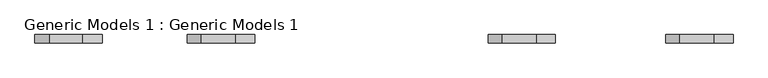
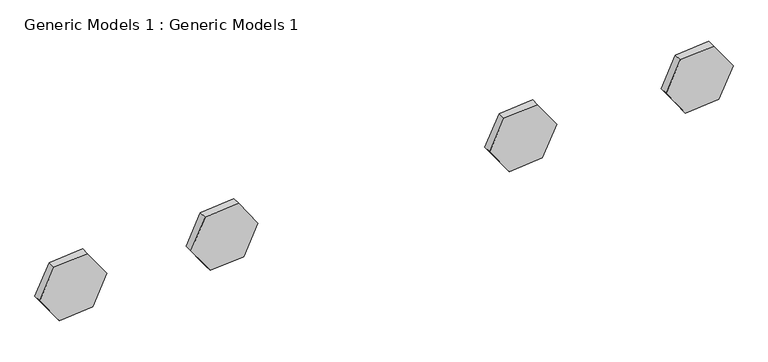
"""IFC4 building model written with IfcOpenShell, lengths in millimetres: proxy geometry, Generic Models 1 : Generic Models 1."""

from ifc_helpers import new_model, si_unit, frame, origin, place, context, project, spatial, polyline, outline, extrude, source, transform, mapped, element, save


def generic_models_1_generic_models_1_2c748ff4(model_context):
    return source(origin(), model_context, "Body", "SweptSolid", [
        extrude(outline(polyline([(1160.0163885, -6657.533371), (607.5311616, -6915.1614634), (108.1760754, -6565.5092678), (161.3062161, -5958.2289798), (713.7914431, -5700.6008875), (1213.1465293, -6050.2530831), (1160.0163885, -6657.533371)])), frame((0.0, -11889.415504, 0.0), z_axis=(0.0, 1.0, 0.0), x_axis=(0.0, 0.0, 1.0)), (0.0, 0.0, 1.0), 152.4),
        extrude(outline(polyline([(1160.0163885, -3914.333371), (607.5311616, -4171.9614634), (108.1760754, -3822.3092678), (161.3062161, -3215.0289798), (713.7914431, -2957.4008875), (1213.1465293, -3307.0530831), (1160.0163885, -3914.333371)])), frame((0.0, -11889.415504, 0.0), z_axis=(0.0, 1.0, 0.0), x_axis=(0.0, 0.0, 1.0)), (0.0, 0.0, 1.0), 152.4),
        extrude(outline(polyline([(1160.0163885, 1506.6435791), (607.5311616, 1249.0154867), (108.1760754, 1598.6676823), (161.3062161, 2205.9479703), (713.7914431, 2463.5760626), (1213.1465293, 2113.923867), (1160.0163885, 1506.6435791)])), frame((0.0, -11889.415504, 0.0), z_axis=(0.0, 1.0, 0.0), x_axis=(0.0, 0.0, 1.0)), (0.0, 0.0, 1.0), 152.4),
        extrude(outline(polyline([(1160.0163885, 4707.0435791), (607.5311616, 4449.4154867), (108.1760754, 4799.0676823), (161.3062161, 5406.3479703), (713.7914431, 5663.9760626), (1213.1465293, 5314.323867), (1160.0163885, 4707.0435791)])), frame((0.0, -11889.415504, 0.0), z_axis=(0.0, 1.0, 0.0), x_axis=(0.0, 0.0, 1.0)), (0.0, 0.0, 1.0), 152.4),
    ])


if __name__ == "__main__":
    model = new_model("IFC4")
    model_context = context("Model", 3, world=origin())
    ifc_project = project(units=[si_unit("LENGTHUNIT", "METRE", prefix="MILLI")], contexts=[model_context])
    site = spatial("IfcSite", under=ifc_project)
    building = spatial("IfcBuilding", under=site)
    placement = place(None, origin())
    generic_models_1_generic_models_1_shape = generic_models_1_generic_models_1_2c748ff4(model_context)
    element("IfcBuildingElementProxy", 1, Name="Generic Models 1 : Generic Models 1", ObjectType="Generic Models 1 : Generic Models 1", at=placement, inside=building, context=model_context, shape_type="MappedRepresentation", body=[
        mapped(generic_models_1_generic_models_1_shape, transform((0.0, 0.0, 0.0), x_axis=(1.0, 0.0, 0.0), y_axis=(0.0, 1.0, 0.0), z_axis=(0.0, 0.0, 1.0))),
    ])
    save(model, "model.ifc")

# Revit data of these elements
# Element 1 (IfcBuildingElementProxy, "Generic Models 1 : Generic Models 1")
#   Materials on its faces: "Parking Stripe"
# Materials
#   "Parking Stripe": class "Paint", colour RGB 250 250 91, transparency 0, Cost = 0
